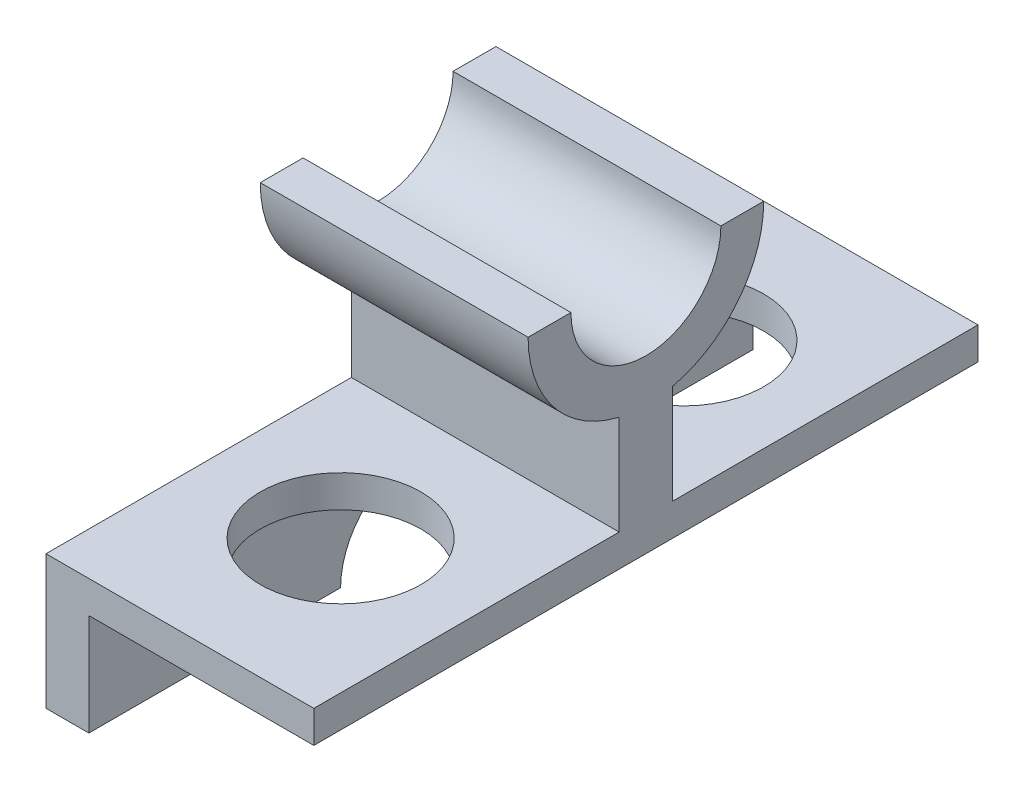
ISO-10303-21;
HEADER;
FILE_DESCRIPTION(('STEP AP214'),'2;1');
FILE_NAME('part.step','',(''),(''),'','','');
FILE_SCHEMA(('AUTOMOTIVE_DESIGN { 1 0 10303 214 1 1 1 1 }'));
ENDSEC;
DATA;
#1=APPLICATION_CONTEXT('core data for automotive mechanical design processes');
#2=APPLICATION_PROTOCOL_DEFINITION('international standard','automotive_design',2000,#1);
#3=PRODUCT_CONTEXT('',#1,'mechanical');
#4=PRODUCT('Part','Part','',(#3));
#5=PRODUCT_RELATED_PRODUCT_CATEGORY('part','',(#4));
#6=PRODUCT_DEFINITION_FORMATION('','',#4);
#7=PRODUCT_DEFINITION_CONTEXT('part definition',#1,'design');
#8=PRODUCT_DEFINITION('design','',#6,#7);
#9=PRODUCT_DEFINITION_SHAPE('','',#8);
#10=(LENGTH_UNIT() NAMED_UNIT(*) SI_UNIT(.MILLI.,.METRE.));
#11=(NAMED_UNIT(*) PLANE_ANGLE_UNIT() SI_UNIT($,.RADIAN.));
#12=(NAMED_UNIT(*) SI_UNIT($,.STERADIAN.) SOLID_ANGLE_UNIT());
#13=UNCERTAINTY_MEASURE_WITH_UNIT(LENGTH_MEASURE(1.E-05),#10,'distance_accuracy_value','');
#14=(GEOMETRIC_REPRESENTATION_CONTEXT(3) GLOBAL_UNCERTAINTY_ASSIGNED_CONTEXT((#13)) GLOBAL_UNIT_ASSIGNED_CONTEXT((#10,
#11,#12)) REPRESENTATION_CONTEXT('',''));
#15=CARTESIAN_POINT('',(0.,0.,0.));
#16=DIRECTION('',(0.,0.,1.));
#17=DIRECTION('',(1.,0.,0.));
#18=AXIS2_PLACEMENT_3D('',#15,#16,#17);
#19=CARTESIAN_POINT('',(0.,0.,124.));
#20=DIRECTION('',(0.,1.,0.));
#21=DIRECTION('',(0.,0.,1.));
#22=AXIS2_PLACEMENT_3D('',#19,#20,#21);
#23=PLANE('',#22);
#24=DIRECTION('',(0.,0.,-1.));
#25=VECTOR('',#24,1.);
#26=CARTESIAN_POINT('',(8.,0.,124.));
#27=LINE('',#26,#25);
#28=CARTESIAN_POINT('',(8.,0.,47.));
#29=VERTEX_POINT('',#28);
#30=CARTESIAN_POINT('',(8.,0.,0.));
#31=VERTEX_POINT('',#30);
#32=EDGE_CURVE('E57',#29,#31,#27,.T.);
#33=ORIENTED_EDGE('',*,*,#32,.F.);
#34=DIRECTION('',(-1.,0.,0.));
#35=VECTOR('',#34,1.);
#36=CARTESIAN_POINT('',(50.,0.,47.));
#37=LINE('',#36,#35);
#38=CARTESIAN_POINT('',(0.,0.,47.));
#39=VERTEX_POINT('',#38);
#40=EDGE_CURVE('E161',#29,#39,#37,.T.);
#41=ORIENTED_EDGE('',*,*,#40,.T.);
#42=DIRECTION('',(0.,0.,-1.));
#43=VECTOR('',#42,1.);
#44=CARTESIAN_POINT('',(0.,0.,124.));
#45=LINE('',#44,#43);
#46=CARTESIAN_POINT('',(0.,0.,0.));
#47=VERTEX_POINT('',#46);
#48=EDGE_CURVE('E175',#39,#47,#45,.T.);
#49=ORIENTED_EDGE('',*,*,#48,.T.);
#50=DIRECTION('',(1.,0.,0.));
#51=VECTOR('',#50,1.);
#52=CARTESIAN_POINT('',(0.,0.,0.));
#53=LINE('',#52,#51);
#54=EDGE_CURVE('E211',#47,#31,#53,.T.);
#55=ORIENTED_EDGE('',*,*,#54,.T.);
#56=EDGE_LOOP('',(#33,#41,#49,#55));
#57=FACE_BOUND('',#56,.T.);
#58=ADVANCED_FACE('F50',(#57),#23,.F.);
#59=CARTESIAN_POINT('',(50.,65.,0.));
#60=DIRECTION('',(0.,1.,0.));
#61=DIRECTION('',(0.,0.,1.));
#62=AXIS2_PLACEMENT_3D('',#59,#60,#61);
#63=PLANE('',#62);
#64=DIRECTION('',(-1.,0.,0.));
#65=VECTOR('',#64,1.);
#66=CARTESIAN_POINT('',(50.,65.,48.));
#67=LINE('',#66,#65);
#68=CARTESIAN_POINT('',(50.,65.,48.));
#69=VERTEX_POINT('',#68);
#70=CARTESIAN_POINT('',(0.,65.,48.));
#71=VERTEX_POINT('',#70);
#72=EDGE_CURVE('E310',#69,#71,#67,.T.);
#73=ORIENTED_EDGE('',*,*,#72,.F.);
#74=DIRECTION('',(0.,0.,-1.));
#75=VECTOR('',#74,1.);
#76=CARTESIAN_POINT('',(50.,65.,0.));
#77=LINE('',#76,#75);
#78=CARTESIAN_POINT('',(50.,65.,40.));
#79=VERTEX_POINT('',#78);
#80=EDGE_CURVE('E287',#69,#79,#77,.T.);
#81=ORIENTED_EDGE('',*,*,#80,.T.);
#82=DIRECTION('',(-1.,0.,0.));
#83=VECTOR('',#82,1.);
#84=CARTESIAN_POINT('',(50.,65.,40.));
#85=LINE('',#84,#83);
#86=CARTESIAN_POINT('',(0.,65.,40.));
#87=VERTEX_POINT('',#86);
#88=EDGE_CURVE('E239',#79,#87,#85,.T.);
#89=ORIENTED_EDGE('',*,*,#88,.T.);
#90=DIRECTION('',(0.,0.,-1.));
#91=VECTOR('',#90,1.);
#92=CARTESIAN_POINT('',(0.,65.,0.));
#93=LINE('',#92,#91);
#94=EDGE_CURVE('E278',#71,#87,#93,.T.);
#95=ORIENTED_EDGE('',*,*,#94,.F.);
#96=EDGE_LOOP('',(#73,#81,#89,#95));
#97=FACE_BOUND('',#96,.T.);
#98=ADVANCED_FACE('F302',(#97),#63,.T.);
#99=CARTESIAN_POINT('',(0.,25.,124.));
#100=DIRECTION('',(0.,-1.,0.));
#101=DIRECTION('',(0.,0.,-1.));
#102=AXIS2_PLACEMENT_3D('',#99,#100,#101);
#103=PLANE('',#102);
#104=CARTESIAN_POINT('',(25.,25.,30.));
#105=DIRECTION('',(0.,-1.,0.));
#106=DIRECTION('',(0.,0.,-1.));
#107=AXIS2_PLACEMENT_3D('',#104,#105,#106);
#108=CIRCLE('',#107,15.);
#109=CARTESIAN_POINT('',(25.,25.,15.));
#110=VERTEX_POINT('',#109);
#111=EDGE_CURVE('E170',#110,#110,#108,.T.);
#112=ORIENTED_EDGE('',*,*,#111,.T.);
#113=EDGE_LOOP('',(#112));
#114=FACE_BOUND('',#113,.T.);
#115=DIRECTION('',(-1.,0.,0.));
#116=VECTOR('',#115,1.);
#117=CARTESIAN_POINT('',(50.,25.,57.));
#118=LINE('',#117,#116);
#119=CARTESIAN_POINT('',(50.,25.,57.));
#120=VERTEX_POINT('',#119);
#121=CARTESIAN_POINT('',(0.,25.,57.));
#122=VERTEX_POINT('',#121);
#123=EDGE_CURVE('E294',#120,#122,#118,.T.);
#124=ORIENTED_EDGE('',*,*,#123,.F.);
#125=DIRECTION('',(0.,0.,-1.));
#126=VECTOR('',#125,1.);
#127=CARTESIAN_POINT('',(50.,25.,124.));
#128=LINE('',#127,#126);
#129=CARTESIAN_POINT('',(50.,25.,0.));
#130=VERTEX_POINT('',#129);
#131=EDGE_CURVE('E194',#120,#130,#128,.T.);
#132=ORIENTED_EDGE('',*,*,#131,.T.);
#133=DIRECTION('',(-1.,0.,0.));
#134=VECTOR('',#133,1.);
#135=CARTESIAN_POINT('',(0.,25.,0.));
#136=LINE('',#135,#134);
#137=CARTESIAN_POINT('',(0.,25.,0.));
#138=VERTEX_POINT('',#137);
#139=EDGE_CURVE('E221',#130,#138,#136,.T.);
#140=ORIENTED_EDGE('',*,*,#139,.T.);
#141=DIRECTION('',(0.,0.,-1.));
#142=VECTOR('',#141,1.);
#143=CARTESIAN_POINT('',(0.,25.,124.));
#144=LINE('',#143,#142);
#145=EDGE_CURVE('E185',#122,#138,#144,.T.);
#146=ORIENTED_EDGE('',*,*,#145,.F.);
#147=EDGE_LOOP('',(#124,#132,#140,#146));
#148=FACE_BOUND('',#147,.T.);
#149=ADVANCED_FACE('F322',(#114,#148),#103,.F.);
#150=CARTESIAN_POINT('',(0.,0.,124.));
#151=VERTEX_POINT('',#150);
#152=CARTESIAN_POINT('',(0.,0.,77.));
#153=VERTEX_POINT('',#152);
#154=EDGE_CURVE('E178',#151,#153,#45,.T.);
#155=ORIENTED_EDGE('',*,*,#154,.T.);
#156=DIRECTION('',(-1.,0.,0.));
#157=VECTOR('',#156,1.);
#158=CARTESIAN_POINT('',(50.,0.,77.));
#159=LINE('',#158,#157);
#160=CARTESIAN_POINT('',(8.,0.,77.));
#161=VERTEX_POINT('',#160);
#162=EDGE_CURVE('E61',#161,#153,#159,.T.);
#163=ORIENTED_EDGE('',*,*,#162,.F.);
#164=CARTESIAN_POINT('',(8.,0.,124.));
#165=VERTEX_POINT('',#164);
#166=EDGE_CURVE('E11',#165,#161,#27,.T.);
#167=ORIENTED_EDGE('',*,*,#166,.F.);
#168=DIRECTION('',(1.,0.,0.));
#169=VECTOR('',#168,1.);
#170=CARTESIAN_POINT('',(0.,0.,124.));
#171=LINE('',#170,#169);
#172=EDGE_CURVE('E229',#151,#165,#171,.T.);
#173=ORIENTED_EDGE('',*,*,#172,.F.);
#174=EDGE_LOOP('',(#155,#163,#167,#173));
#175=FACE_BOUND('',#174,.T.);
#176=ADVANCED_FACE('F47',(#175),#23,.F.);
#177=CARTESIAN_POINT('',(8.,19.,124.));
#178=DIRECTION('',(-1.,0.,0.));
#179=DIRECTION('',(0.,0.,1.));
#180=AXIS2_PLACEMENT_3D('',#177,#178,#179);
#181=PLANE('',#180);
#182=ORIENTED_EDGE('',*,*,#166,.T.);
#183=CARTESIAN_POINT('',(8.,0.,62.));
#184=DIRECTION('',(-1.,0.,0.));
#185=DIRECTION('',(0.,0.,1.));
#186=AXIS2_PLACEMENT_3D('',#183,#184,#185);
#187=CIRCLE('',#186,15.);
#188=EDGE_CURVE('E208',#161,#29,#187,.T.);
#189=ORIENTED_EDGE('',*,*,#188,.T.);
#190=ORIENTED_EDGE('',*,*,#32,.T.);
#191=DIRECTION('',(0.,1.,0.));
#192=VECTOR('',#191,1.);
#193=CARTESIAN_POINT('',(8.,19.,0.));
#194=LINE('',#193,#192);
#195=CARTESIAN_POINT('',(8.,19.,0.));
#196=VERTEX_POINT('',#195);
#197=EDGE_CURVE('E210',#31,#196,#194,.T.);
#198=ORIENTED_EDGE('',*,*,#197,.T.);
#199=DIRECTION('',(0.,0.,-1.));
#200=VECTOR('',#199,1.);
#201=CARTESIAN_POINT('',(8.,19.,124.));
#202=LINE('',#201,#200);
#203=CARTESIAN_POINT('',(8.,19.,124.));
#204=VERTEX_POINT('',#203);
#205=EDGE_CURVE('E196',#204,#196,#202,.T.);
#206=ORIENTED_EDGE('',*,*,#205,.F.);
#207=DIRECTION('',(0.,1.,0.));
#208=VECTOR('',#207,1.);
#209=CARTESIAN_POINT('',(8.,19.,124.));
#210=LINE('',#209,#208);
#211=EDGE_CURVE('E234',#165,#204,#210,.T.);
#212=ORIENTED_EDGE('',*,*,#211,.F.);
#213=EDGE_LOOP('',(#182,#189,#190,#198,#206,#212));
#214=FACE_BOUND('',#213,.T.);
#215=ADVANCED_FACE('F206',(#214),#181,.F.);
#216=CARTESIAN_POINT('',(50.,19.,124.));
#217=DIRECTION('',(0.,1.,0.));
#218=DIRECTION('',(0.,0.,1.));
#219=AXIS2_PLACEMENT_3D('',#216,#217,#218);
#220=PLANE('',#219);
#221=CARTESIAN_POINT('',(25.,19.,94.));
#222=DIRECTION('',(0.,-1.,0.));
#223=DIRECTION('',(0.,0.,-1.));
#224=AXIS2_PLACEMENT_3D('',#221,#222,#223);
#225=CIRCLE('',#224,15.);
#226=CARTESIAN_POINT('',(25.,19.,79.));
#227=VERTEX_POINT('',#226);
#228=EDGE_CURVE('E593',#227,#227,#225,.T.);
#229=ORIENTED_EDGE('',*,*,#228,.F.);
#230=EDGE_LOOP('',(#229));
#231=FACE_BOUND('',#230,.T.);
#232=CARTESIAN_POINT('',(25.,19.,30.));
#233=DIRECTION('',(0.,-1.,0.));
#234=DIRECTION('',(0.,0.,-1.));
#235=AXIS2_PLACEMENT_3D('',#232,#233,#234);
#236=CIRCLE('',#235,15.);
#237=CARTESIAN_POINT('',(25.,19.,15.));
#238=VERTEX_POINT('',#237);
#239=EDGE_CURVE('E589',#238,#238,#236,.T.);
#240=ORIENTED_EDGE('',*,*,#239,.F.);
#241=EDGE_LOOP('',(#240));
#242=FACE_BOUND('',#241,.T.);
#243=DIRECTION('',(1.,0.,0.));
#244=VECTOR('',#243,1.);
#245=CARTESIAN_POINT('',(50.,19.,0.));
#246=LINE('',#245,#244);
#247=CARTESIAN_POINT('',(50.,19.,0.));
#248=VERTEX_POINT('',#247);
#249=EDGE_CURVE('E213',#196,#248,#246,.T.);
#250=ORIENTED_EDGE('',*,*,#249,.T.);
#251=DIRECTION('',(0.,0.,-1.));
#252=VECTOR('',#251,1.);
#253=CARTESIAN_POINT('',(50.,19.,124.));
#254=LINE('',#253,#252);
#255=CARTESIAN_POINT('',(50.,19.,124.));
#256=VERTEX_POINT('',#255);
#257=EDGE_CURVE('E192',#256,#248,#254,.T.);
#258=ORIENTED_EDGE('',*,*,#257,.F.);
#259=DIRECTION('',(1.,0.,0.));
#260=VECTOR('',#259,1.);
#261=CARTESIAN_POINT('',(50.,19.,124.));
#262=LINE('',#261,#260);
#263=EDGE_CURVE('E237',#204,#256,#262,.T.);
#264=ORIENTED_EDGE('',*,*,#263,.F.);
#265=ORIENTED_EDGE('',*,*,#205,.T.);
#266=EDGE_LOOP('',(#250,#258,#264,#265));
#267=FACE_BOUND('',#266,.T.);
#268=ADVANCED_FACE('F260',(#231,#242,#267),#220,.F.);
#269=CARTESIAN_POINT('',(50.,25.,124.));
#270=DIRECTION('',(-1.,0.,0.));
#271=DIRECTION('',(0.,0.,1.));
#272=AXIS2_PLACEMENT_3D('',#269,#270,#271);
#273=PLANE('',#272);
#274=ORIENTED_EDGE('',*,*,#80,.F.);
#275=CARTESIAN_POINT('',(50.,65.,62.));
#276=DIRECTION('',(-1.,0.,0.));
#277=DIRECTION('',(0.,0.,1.));
#278=AXIS2_PLACEMENT_3D('',#275,#276,#277);
#279=CIRCLE('',#278,14.);
#280=CARTESIAN_POINT('',(50.,65.,76.));
#281=VERTEX_POINT('',#280);
#282=EDGE_CURVE('E315',#69,#281,#279,.T.);
#283=ORIENTED_EDGE('',*,*,#282,.T.);
#284=CARTESIAN_POINT('',(50.,65.,84.));
#285=VERTEX_POINT('',#284);
#286=EDGE_CURVE('E320',#285,#281,#77,.T.);
#287=ORIENTED_EDGE('',*,*,#286,.F.);
#288=CARTESIAN_POINT('',(50.,65.,62.));
#289=DIRECTION('',(-1.,0.,0.));
#290=DIRECTION('',(0.,0.,1.));
#291=AXIS2_PLACEMENT_3D('',#288,#289,#290);
#292=CIRCLE('',#291,22.);
#293=CARTESIAN_POINT('',(50.,43.5757147143715,67.));
#294=VERTEX_POINT('',#293);
#295=EDGE_CURVE('E270',#294,#285,#292,.T.);
#296=ORIENTED_EDGE('',*,*,#295,.F.);
#297=DIRECTION('',(0.,1.,0.));
#298=VECTOR('',#297,1.);
#299=CARTESIAN_POINT('',(50.,0.,67.));
#300=LINE('',#299,#298);
#301=CARTESIAN_POINT('',(50.,25.,67.));
#302=VERTEX_POINT('',#301);
#303=EDGE_CURVE('E262',#302,#294,#300,.T.);
#304=ORIENTED_EDGE('',*,*,#303,.F.);
#305=CARTESIAN_POINT('',(50.,25.,124.));
#306=VERTEX_POINT('',#305);
#307=EDGE_CURVE('E191',#306,#302,#128,.T.);
#308=ORIENTED_EDGE('',*,*,#307,.F.);
#309=DIRECTION('',(0.,1.,0.));
#310=VECTOR('',#309,1.);
#311=CARTESIAN_POINT('',(50.,25.,124.));
#312=LINE('',#311,#310);
#313=EDGE_CURVE('E241',#256,#306,#312,.T.);
#314=ORIENTED_EDGE('',*,*,#313,.F.);
#315=ORIENTED_EDGE('',*,*,#257,.T.);
#316=DIRECTION('',(0.,1.,0.));
#317=VECTOR('',#316,1.);
#318=CARTESIAN_POINT('',(50.,25.,0.));
#319=LINE('',#318,#317);
#320=EDGE_CURVE('E225',#248,#130,#319,.T.);
#321=ORIENTED_EDGE('',*,*,#320,.T.);
#322=ORIENTED_EDGE('',*,*,#131,.F.);
#323=DIRECTION('',(0.,1.,0.));
#324=VECTOR('',#323,1.);
#325=CARTESIAN_POINT('',(50.,0.,57.));
#326=LINE('',#325,#324);
#327=CARTESIAN_POINT('',(50.,43.5757147143715,57.));
#328=VERTEX_POINT('',#327);
#329=EDGE_CURVE('E267',#120,#328,#326,.T.);
#330=ORIENTED_EDGE('',*,*,#329,.T.);
#331=CARTESIAN_POINT('',(50.,65.,62.));
#332=DIRECTION('',(-1.,0.,0.));
#333=DIRECTION('',(0.,0.,1.));
#334=AXIS2_PLACEMENT_3D('',#331,#332,#333);
#335=CIRCLE('',#334,22.);
#336=EDGE_CURVE('E275',#79,#328,#335,.T.);
#337=ORIENTED_EDGE('',*,*,#336,.F.);
#338=EDGE_LOOP('',(#274,#283,#287,#296,#304,#308,#314,#315,#321,#322,#330,#337));
#339=FACE_BOUND('',#338,.T.);
#340=ADVANCED_FACE('F257',(#339),#273,.F.);
#341=CARTESIAN_POINT('',(25.,25.,94.));
#342=DIRECTION('',(0.,-1.,0.));
#343=DIRECTION('',(0.,0.,-1.));
#344=AXIS2_PLACEMENT_3D('',#341,#342,#343);
#345=CIRCLE('',#344,15.);
#346=CARTESIAN_POINT('',(25.,25.,79.));
#347=VERTEX_POINT('',#346);
#348=EDGE_CURVE('E51',#347,#347,#345,.T.);
#349=ORIENTED_EDGE('',*,*,#348,.T.);
#350=EDGE_LOOP('',(#349));
#351=FACE_BOUND('',#350,.T.);
#352=ORIENTED_EDGE('',*,*,#307,.T.);
#353=DIRECTION('',(-1.,0.,0.));
#354=VECTOR('',#353,1.);
#355=CARTESIAN_POINT('',(50.,25.,67.));
#356=LINE('',#355,#354);
#357=CARTESIAN_POINT('',(0.,25.,67.));
#358=VERTEX_POINT('',#357);
#359=EDGE_CURVE('E251',#302,#358,#356,.T.);
#360=ORIENTED_EDGE('',*,*,#359,.T.);
#361=CARTESIAN_POINT('',(0.,25.,124.));
#362=VERTEX_POINT('',#361);
#363=EDGE_CURVE('E186',#362,#358,#144,.T.);
#364=ORIENTED_EDGE('',*,*,#363,.F.);
#365=DIRECTION('',(-1.,0.,0.));
#366=VECTOR('',#365,1.);
#367=CARTESIAN_POINT('',(0.,25.,124.));
#368=LINE('',#367,#366);
#369=EDGE_CURVE('E181',#306,#362,#368,.T.);
#370=ORIENTED_EDGE('',*,*,#369,.F.);
#371=EDGE_LOOP('',(#352,#360,#364,#370));
#372=FACE_BOUND('',#371,.T.);
#373=ADVANCED_FACE('F252',(#351,#372),#103,.F.);
#374=CARTESIAN_POINT('',(0.,0.,124.));
#375=DIRECTION('',(1.,0.,0.));
#376=DIRECTION('',(0.,0.,-1.));
#377=AXIS2_PLACEMENT_3D('',#374,#375,#376);
#378=PLANE('',#377);
#379=ORIENTED_EDGE('',*,*,#48,.F.);
#380=CARTESIAN_POINT('',(0.,0.,62.));
#381=DIRECTION('',(-1.,0.,0.));
#382=DIRECTION('',(0.,0.,1.));
#383=AXIS2_PLACEMENT_3D('',#380,#381,#382);
#384=CIRCLE('',#383,15.);
#385=EDGE_CURVE('E158',#153,#39,#384,.T.);
#386=ORIENTED_EDGE('',*,*,#385,.F.);
#387=ORIENTED_EDGE('',*,*,#154,.F.);
#388=DIRECTION('',(0.,-1.,0.));
#389=VECTOR('',#388,1.);
#390=CARTESIAN_POINT('',(0.,0.,124.));
#391=LINE('',#390,#389);
#392=EDGE_CURVE('E177',#362,#151,#391,.T.);
#393=ORIENTED_EDGE('',*,*,#392,.F.);
#394=ORIENTED_EDGE('',*,*,#363,.T.);
#395=DIRECTION('',(0.,1.,0.));
#396=VECTOR('',#395,1.);
#397=CARTESIAN_POINT('',(0.,0.,67.));
#398=LINE('',#397,#396);
#399=CARTESIAN_POINT('',(0.,43.5757147143715,67.));
#400=VERTEX_POINT('',#399);
#401=EDGE_CURVE('E289',#358,#400,#398,.T.);
#402=ORIENTED_EDGE('',*,*,#401,.T.);
#403=CARTESIAN_POINT('',(0.,65.,62.));
#404=DIRECTION('',(-1.,0.,0.));
#405=DIRECTION('',(0.,0.,1.));
#406=AXIS2_PLACEMENT_3D('',#403,#404,#405);
#407=CIRCLE('',#406,22.);
#408=CARTESIAN_POINT('',(0.,65.,84.));
#409=VERTEX_POINT('',#408);
#410=EDGE_CURVE('E290',#400,#409,#407,.T.);
#411=ORIENTED_EDGE('',*,*,#410,.T.);
#412=CARTESIAN_POINT('',(0.,65.,76.));
#413=VERTEX_POINT('',#412);
#414=EDGE_CURVE('E277',#409,#413,#93,.T.);
#415=ORIENTED_EDGE('',*,*,#414,.T.);
#416=CARTESIAN_POINT('',(0.,65.,62.));
#417=DIRECTION('',(-1.,0.,0.));
#418=DIRECTION('',(0.,0.,1.));
#419=AXIS2_PLACEMENT_3D('',#416,#417,#418);
#420=CIRCLE('',#419,14.);
#421=EDGE_CURVE('E72',#71,#413,#420,.T.);
#422=ORIENTED_EDGE('',*,*,#421,.F.);
#423=ORIENTED_EDGE('',*,*,#94,.T.);
#424=CARTESIAN_POINT('',(0.,65.,62.));
#425=DIRECTION('',(-1.,0.,0.));
#426=DIRECTION('',(0.,0.,1.));
#427=AXIS2_PLACEMENT_3D('',#424,#425,#426);
#428=CIRCLE('',#427,22.);
#429=CARTESIAN_POINT('',(0.,43.5757147143715,57.));
#430=VERTEX_POINT('',#429);
#431=EDGE_CURVE('E276',#87,#430,#428,.T.);
#432=ORIENTED_EDGE('',*,*,#431,.T.);
#433=DIRECTION('',(0.,1.,0.));
#434=VECTOR('',#433,1.);
#435=CARTESIAN_POINT('',(0.,0.,57.));
#436=LINE('',#435,#434);
#437=EDGE_CURVE('E281',#122,#430,#436,.T.);
#438=ORIENTED_EDGE('',*,*,#437,.F.);
#439=ORIENTED_EDGE('',*,*,#145,.T.);
#440=DIRECTION('',(0.,-1.,0.));
#441=VECTOR('',#440,1.);
#442=CARTESIAN_POINT('',(0.,0.,0.));
#443=LINE('',#442,#441);
#444=EDGE_CURVE('E176',#138,#47,#443,.T.);
#445=ORIENTED_EDGE('',*,*,#444,.T.);
#446=EDGE_LOOP('',(#379,#386,#387,#393,#394,#402,#411,#415,#422,#423,#432,#438,#439,#445));
#447=FACE_BOUND('',#446,.T.);
#448=ADVANCED_FACE('F172',(#447),#378,.F.);
#449=CARTESIAN_POINT('',(0.,0.,124.));
#450=DIRECTION('',(0.,0.,-1.));
#451=DIRECTION('',(-1.,0.,0.));
#452=AXIS2_PLACEMENT_3D('',#449,#450,#451);
#453=PLANE('',#452);
#454=ORIENTED_EDGE('',*,*,#172,.T.);
#455=ORIENTED_EDGE('',*,*,#211,.T.);
#456=ORIENTED_EDGE('',*,*,#263,.T.);
#457=ORIENTED_EDGE('',*,*,#313,.T.);
#458=ORIENTED_EDGE('',*,*,#369,.T.);
#459=ORIENTED_EDGE('',*,*,#392,.T.);
#460=EDGE_LOOP('',(#454,#455,#456,#457,#458,#459));
#461=FACE_BOUND('',#460,.T.);
#462=ADVANCED_FACE('F249',(#461),#453,.F.);
#463=CARTESIAN_POINT('',(0.,0.,0.));
#464=DIRECTION('',(0.,0.,-1.));
#465=DIRECTION('',(-1.,0.,0.));
#466=AXIS2_PLACEMENT_3D('',#463,#464,#465);
#467=PLANE('',#466);
#468=ORIENTED_EDGE('',*,*,#54,.F.);
#469=ORIENTED_EDGE('',*,*,#444,.F.);
#470=ORIENTED_EDGE('',*,*,#139,.F.);
#471=ORIENTED_EDGE('',*,*,#320,.F.);
#472=ORIENTED_EDGE('',*,*,#249,.F.);
#473=ORIENTED_EDGE('',*,*,#197,.F.);
#474=EDGE_LOOP('',(#468,#469,#470,#471,#472,#473));
#475=FACE_BOUND('',#474,.T.);
#476=ADVANCED_FACE('F209',(#475),#467,.T.);
#477=DIRECTION('',(-1.,0.,0.));
#478=VECTOR('',#477,1.);
#479=CARTESIAN_POINT('',(50.,65.,76.));
#480=LINE('',#479,#478);
#481=EDGE_CURVE('E309',#281,#413,#480,.T.);
#482=ORIENTED_EDGE('',*,*,#481,.T.);
#483=ORIENTED_EDGE('',*,*,#414,.F.);
#484=DIRECTION('',(-1.,0.,0.));
#485=VECTOR('',#484,1.);
#486=CARTESIAN_POINT('',(50.,65.,84.));
#487=LINE('',#486,#485);
#488=EDGE_CURVE('E214',#285,#409,#487,.T.);
#489=ORIENTED_EDGE('',*,*,#488,.F.);
#490=ORIENTED_EDGE('',*,*,#286,.T.);
#491=EDGE_LOOP('',(#482,#483,#489,#490));
#492=FACE_BOUND('',#491,.T.);
#493=ADVANCED_FACE('F334',(#492),#63,.T.);
#494=CARTESIAN_POINT('',(50.,65.,62.));
#495=DIRECTION('',(-1.,0.,0.));
#496=DIRECTION('',(0.,0.,1.));
#497=AXIS2_PLACEMENT_3D('',#494,#495,#496);
#498=CYLINDRICAL_SURFACE('',#497,22.);
#499=ORIENTED_EDGE('',*,*,#410,.F.);
#500=DIRECTION('',(-1.,0.,0.));
#501=VECTOR('',#500,1.);
#502=CARTESIAN_POINT('',(50.,43.5757147143715,67.));
#503=LINE('',#502,#501);
#504=EDGE_CURVE('E220',#294,#400,#503,.T.);
#505=ORIENTED_EDGE('',*,*,#504,.F.);
#506=ORIENTED_EDGE('',*,*,#295,.T.);
#507=ORIENTED_EDGE('',*,*,#488,.T.);
#508=EDGE_LOOP('',(#499,#505,#506,#507));
#509=FACE_BOUND('',#508,.T.);
#510=ADVANCED_FACE('F423',(#509),#498,.T.);
#511=CARTESIAN_POINT('',(50.,0.,67.));
#512=DIRECTION('',(0.,0.,1.));
#513=DIRECTION('',(1.,0.,0.));
#514=AXIS2_PLACEMENT_3D('',#511,#512,#513);
#515=PLANE('',#514);
#516=ORIENTED_EDGE('',*,*,#401,.F.);
#517=ORIENTED_EDGE('',*,*,#359,.F.);
#518=ORIENTED_EDGE('',*,*,#303,.T.);
#519=ORIENTED_EDGE('',*,*,#504,.T.);
#520=EDGE_LOOP('',(#516,#517,#518,#519));
#521=FACE_BOUND('',#520,.T.);
#522=ADVANCED_FACE('F429',(#521),#515,.T.);
#523=CARTESIAN_POINT('',(50.,0.,57.));
#524=DIRECTION('',(0.,0.,1.));
#525=DIRECTION('',(1.,0.,0.));
#526=AXIS2_PLACEMENT_3D('',#523,#524,#525);
#527=PLANE('',#526);
#528=ORIENTED_EDGE('',*,*,#437,.T.);
#529=DIRECTION('',(-1.,0.,0.));
#530=VECTOR('',#529,1.);
#531=CARTESIAN_POINT('',(50.,43.5757147143715,57.));
#532=LINE('',#531,#530);
#533=EDGE_CURVE('E293',#328,#430,#532,.T.);
#534=ORIENTED_EDGE('',*,*,#533,.F.);
#535=ORIENTED_EDGE('',*,*,#329,.F.);
#536=ORIENTED_EDGE('',*,*,#123,.T.);
#537=EDGE_LOOP('',(#528,#534,#535,#536));
#538=FACE_BOUND('',#537,.T.);
#539=ADVANCED_FACE('F323',(#538),#527,.F.);
#540=CARTESIAN_POINT('',(50.,65.,62.));
#541=DIRECTION('',(-1.,0.,0.));
#542=DIRECTION('',(0.,0.,1.));
#543=AXIS2_PLACEMENT_3D('',#540,#541,#542);
#544=CYLINDRICAL_SURFACE('',#543,22.);
#545=ORIENTED_EDGE('',*,*,#431,.F.);
#546=ORIENTED_EDGE('',*,*,#88,.F.);
#547=ORIENTED_EDGE('',*,*,#336,.T.);
#548=ORIENTED_EDGE('',*,*,#533,.T.);
#549=EDGE_LOOP('',(#545,#546,#547,#548));
#550=FACE_BOUND('',#549,.T.);
#551=ADVANCED_FACE('F307',(#550),#544,.T.);
#552=CARTESIAN_POINT('',(50.,65.,62.));
#553=DIRECTION('',(-1.,0.,0.));
#554=DIRECTION('',(0.,0.,1.));
#555=AXIS2_PLACEMENT_3D('',#552,#553,#554);
#556=CYLINDRICAL_SURFACE('',#555,14.);
#557=ORIENTED_EDGE('',*,*,#421,.T.);
#558=ORIENTED_EDGE('',*,*,#481,.F.);
#559=ORIENTED_EDGE('',*,*,#282,.F.);
#560=ORIENTED_EDGE('',*,*,#72,.T.);
#561=EDGE_LOOP('',(#557,#558,#559,#560));
#562=FACE_BOUND('',#561,.T.);
#563=ADVANCED_FACE('F452',(#562),#556,.F.);
#564=CARTESIAN_POINT('',(50.,0.,62.));
#565=DIRECTION('',(-1.,0.,0.));
#566=DIRECTION('',(0.,0.,1.));
#567=AXIS2_PLACEMENT_3D('',#564,#565,#566);
#568=CYLINDRICAL_SURFACE('',#567,15.);
#569=ORIENTED_EDGE('',*,*,#162,.T.);
#570=ORIENTED_EDGE('',*,*,#385,.T.);
#571=ORIENTED_EDGE('',*,*,#40,.F.);
#572=ORIENTED_EDGE('',*,*,#188,.F.);
#573=EDGE_LOOP('',(#569,#570,#571,#572));
#574=FACE_BOUND('',#573,.T.);
#575=ADVANCED_FACE('F159',(#574),#568,.F.);
#576=CARTESIAN_POINT('',(25.,39.,94.));
#577=DIRECTION('',(0.,-1.,0.));
#578=DIRECTION('',(0.,0.,-1.));
#579=AXIS2_PLACEMENT_3D('',#576,#577,#578);
#580=CYLINDRICAL_SURFACE('',#579,15.);
#581=ORIENTED_EDGE('',*,*,#228,.T.);
#582=EDGE_LOOP('',(#581));
#583=FACE_BOUND('',#582,.T.);
#584=ORIENTED_EDGE('',*,*,#348,.F.);
#585=EDGE_LOOP('',(#584));
#586=FACE_BOUND('',#585,.T.);
#587=ADVANCED_FACE('F467',(#583,#586),#580,.F.);
#588=CARTESIAN_POINT('',(25.,39.,30.));
#589=DIRECTION('',(0.,-1.,0.));
#590=DIRECTION('',(0.,0.,-1.));
#591=AXIS2_PLACEMENT_3D('',#588,#589,#590);
#592=CYLINDRICAL_SURFACE('',#591,15.);
#593=ORIENTED_EDGE('',*,*,#239,.T.);
#594=EDGE_LOOP('',(#593));
#595=FACE_BOUND('',#594,.T.);
#596=ORIENTED_EDGE('',*,*,#111,.F.);
#597=EDGE_LOOP('',(#596));
#598=FACE_BOUND('',#597,.T.);
#599=ADVANCED_FACE('F476',(#595,#598),#592,.F.);
#600=CLOSED_SHELL('',(#58,#98,#149,#176,#215,#268,#340,#373,#448,#462,#476,#493,#510,#522,#539,
#551,#563,#575,#587,#599));
#601=MANIFOLD_SOLID_BREP('B2',#600);
#602=ADVANCED_BREP_SHAPE_REPRESENTATION('',(#18,#601),#14);
#603=SHAPE_DEFINITION_REPRESENTATION(#9,#602);
ENDSEC;
END-ISO-10303-21;
